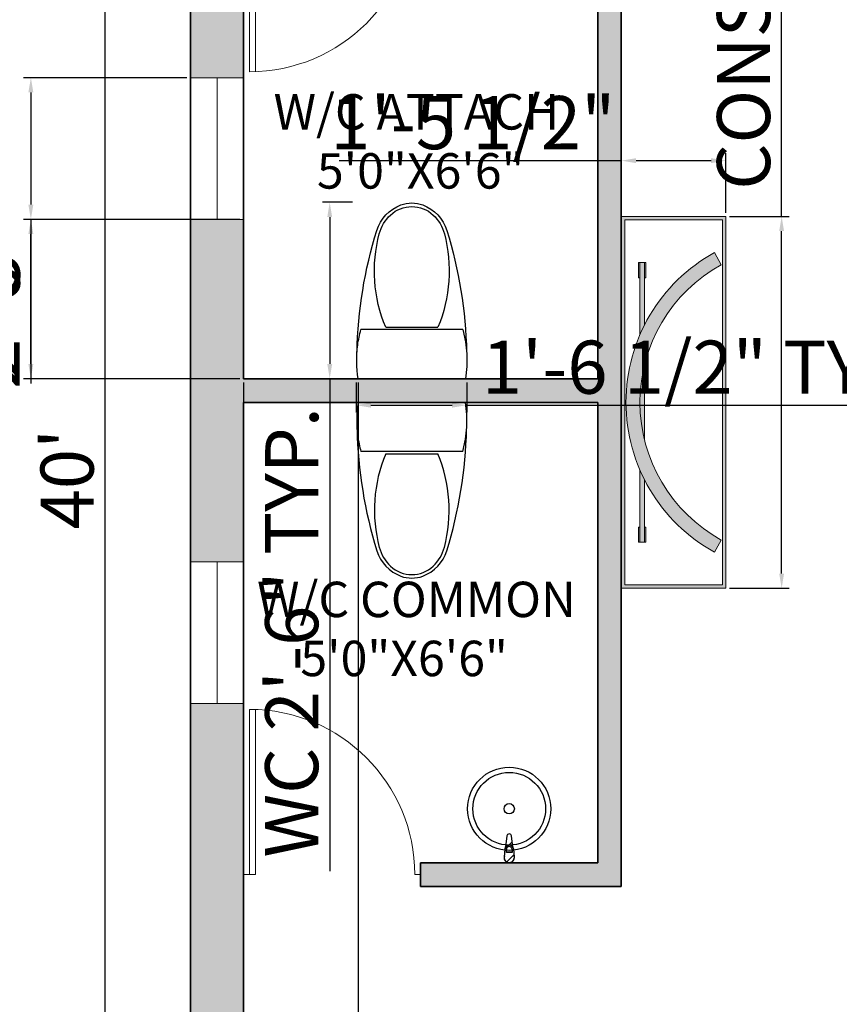
# Model space of a CAD drawing. Units: inches. Extents: x 3592 to 4861, y 1650 to 2243.
# Tile 3 of 30: x 4009 to 4148, y 1836 to 2003. Entities that reach past the tile are written whole.
import ezdxf

# ---------------------------------------------------------------- set-up
doc = ezdxf.new("R2010")
doc.units = ezdxf.units.IN
for name, color, linetype, lineweight in [('A-ANNO-DIMS', 2, 'Continuous', 13), ('A-AREA-IDEN', 7, 'Continuous', 18), ('A-DOOR', 3, 'Continuous', 20), ('A-FURN', 9, 'Continuous', 13), ('A-GLAZ', 4, 'Continuous', 18), ('A-WALL', 7, 'Continuous', 35), ('aparador', 36, 'Continuous', 9), ('moveis', 254, 'Continuous', 5), ('Сантехника', 9, 'Continuous', 18)]:
    doc.layers.add(name, color=color, linetype=linetype, lineweight=lineweight)
doc.layers.add('A-WALL-PATT', color=252, linetype='Continuous', lineweight=13, true_color=0x939598)
doc.layers.add('SANTEH', color=7, linetype='Continuous')
doc.styles.get("Standard").update_dxf_attribs({"font": 'arial.ttf'})
doc.dimstyles.new('ISO-25', dxfattribs={"dimtxt": 9, "dimasz": 2.5, "dimexe": 1.25, "dimexo": 0.625, "dimtad": 1, "dimlunit": 3, "dimtxsty": 'Standard', "dimcen": 2.5, "dimadec": 0, "dimazin": 0, "dimtfac": 1, "dimtmove": 0, "dimatfit": 3, "dimfxl": 1, "dimarcsym": 0})
pattern_1 = [(45, (-0.056, -259.036), (-35.355, 35.355), [])]

# ---------------------------------------------------------------- blocks, each defined once
blk = doc.blocks.new('2')
for p, q in [((3637.19, 1914.49), (3637.19, 1942.49)), ((3638.19, 1914.49), (3638.19, 1942.49)), ((3636.19, 1914.49), (3638.19, 1914.49)), ((3665.19, 1914.49), (3666.19, 1914.49))]:
    blk.add_line(p, q)
blk.add_arc((3637.19, 1914.49), 28, 0, 90)
blk = doc.blocks.new('*D6')
at = {"layer": 'A-ANNO-DIMS', "color": 0, "lineweight": -2, "transparency": 16777216}
for p, q in [((4037.74, 2165.22), (4022.59, 2165.22)), ((4023.84, 2162.72), (4023.84, 1687.72)), ((4037.74, 1685.22), (4022.59, 1685.22))]:
    blk.add_line(p, q, dxfattribs=at)
at = {"layer": 'A-ANNO-DIMS', "color": 0, "transparency": 16777216}
for points in [[(4023.43, 2162.72), (4024.26, 2162.72), (4023.84, 2165.22)], [(4023.43, 1687.72), (4024.26, 1687.72), (4023.84, 1685.22)]]:
    blk.add_solid(points, dxfattribs=at)
at = {"layer": 'Defpoints', "color": 0, "transparency": 16777216}
for p in [(4038.37, 2165.22), (4023.84, 1685.22), (4038.37, 1685.22)]:
    blk.add_point(p, dxfattribs=at)
at = {"layer": 'A-ANNO-DIMS', "color": 0, "transparency": 16777216, "insert": (4018.62, 1925.22), "char_height": 9, "attachment_point": 5, "rotation": 90}
blk.add_mtext("40'", dxfattribs=at)
blk = doc.blocks.new('r13')
at = {"layer": 'SANTEH', "ltscale": 5}
h = blk.add_hatch(dxfattribs=at)
h.set_pattern_fill('100__1', color=256, scale=0.5, angle=45, style=0)
h.set_pattern_definition(pattern_1)
h.paths.add_polyline_path([(-0.1, -138.2, -0.378173), (-11.2, -128.4), (-17.8, -75.5, -0.12102), (-21.1, -66), (-23.4, -32.9, -0.524536), (-0.1, 1)], flags=0)
h = blk.add_hatch(dxfattribs=at)
h.set_pattern_fill('100__1', color=256, scale=0.5, angle=45, style=0)
h.set_pattern_definition(pattern_1)
h.paths.add_polyline_path([(-0.1, -138.2, 0.378173), (11, -128.4), (17.7, -75.5, 0.12102), (20.9, -66), (23.3, -32.9, 0.524536), (-0.1, 1)], flags=0)
for p, q in [((-24, -25.7), (-23.9, -20.6)), ((-21.1, -66), (-24, -25.7)), ((20.9, -66), (23.8, -25.7)), ((23.8, -25.7), (23.8, -20.7)), ((-17.8, -75.5), (-11.2, -128.4)), ((-13.7, -48.9), (13.5, -48.9)), ((-13.7, -63.8), (-13.7, -48.9)), ((-13.7, -49.6), (13.5, -49.6)), ((11, -128.4), (17.7, -75.5)), ((13.5, -48.9), (13.5, -63.8))]:
    blk.add_line(p, q, dxfattribs=at)
for radius in [200, 175, 25]:
    blk.add_circle((-0.1, -259), radius, dxfattribs=at)
for centre, radius, start, end in [((-0.1, -24), 25, 339.2856, 200.7144), ((-0.1, -24), 24, 7.8374, 171.8967), ((-0.1, -63.4), 21.1, 185.1696, 354.8304), ((-0.1, -64.1), 21.1, 185.1696, 354.8304), ((-0.1, -63.8), 13.6, 180, 0), ((-0.1, -127), 11.2, 187.1389, 352.8611)]:
    blk.add_arc(centre, radius, start, end, dxfattribs=at)
blk = doc.blocks.new('y5')
at = {"layer": 'SANTEH', "ltscale": 5}
for p, q in [((392.5, 0), (0, 0)), ((382.5, -180), (10, -180)), ((100.6, -188.2), (291.9, -188.2))]:
    blk.add_line(p, q, dxfattribs=at)
blk.add_lwpolyline([(382.5, -180), (392.6, -134.7), (397.5, -90.9), (397.5, -44.6), (392.5, 0)], dxfattribs=at)
for centre, radius, start, end in [((406.3, -67.7), 411.9, 170.5377, 187.7399), ((1615.7, -62.7), 1620.4, 181.2224, 197.2477), ((-1223.2, -62.7), 1620.4, 342.7523, 358.7776), ((406.3, -67.7), 411.9, 187.7399, 195.822), ((594.7, -394.2), 535.3, 157.3737, 194.7786), ((-202.2, -394.2), 535.3, 345.2214, 22.6263), ((216.9, -493.8), 144.6, 194.7786, 226.8543), ((175.6, -493.8), 144.6, 313.1457, 345.2214), ((207.1, -500), 145.4, 197.2477, 249.5476), ((185.4, -500), 145.4, 290.4524, 342.7523), ((196.3, -515.9), 114.4, 226.8543, 313.1457), ((196.3, -529), 114.4, 249.5476, 290.4524)]:
    blk.add_arc(centre, radius, start, end, dxfattribs=at)
blk = doc.blocks.new('Aparador ORGANICA Formatto')
at = {"layer": 'aparador', "ltscale": 0.3}
h = blk.add_hatch(color=256, dxfattribs=at)
h.dxf.hatch_style = 1
h.set_gradient(color1=(118, 213, 123), color2=(52, 168, 57), one_color=1, tint=0.43, name='INVCURVED')
h.paths.add_polyline_path([(0.8, 0.45), (-0.8, 0.45), (-0.8, 0), (0.8, 0)])
h.paths.add_polyline_path([(0.785, 0.435), (0.785, 0.015), (-0.785, 0.015), (-0.785, 0.435)], flags=16)
h.paths.add_polyline_path([(0.2911, 0.3699), (0.5365, 0.3699), (0.5365, 0.3757), (0.6011, 0.3757), (0.6011, 0.3699), (0.6011, 0.3499), (0.6011, 0.3441), (0.5365, 0.3441), (0.5365, 0.3499), (0.3338, 0.3499, -0.150336), (0.6449, 0.0488), (0.5923, 0.0199, 0.208852), (0.1632, 0.3499), (-0.1632, 0.3499, 0.208852), (-0.5923, 0.0199), (-0.6449, 0.0488, -0.150336), (-0.3338, 0.3499), (-0.5365, 0.3499), (-0.5365, 0.3441), (-0.6011, 0.3441), (-0.6011, 0.3499), (-0.6011, 0.3699), (-0.6011, 0.3757), (-0.5365, 0.3757), (-0.5365, 0.3699), (-0.2911, 0.3699, -0.206106)], flags=0)
h = blk.add_hatch(color=256, dxfattribs=at)
h.dxf.hatch_style = 1
h.set_gradient(color1=(135, 92, 69), color2=(0, 0, 0), one_color=1, name='INVCURVED')
h.paths.add_polyline_path([(-0.6449, 0.0488), (-0.5923, 0.0199, -0.590888), (0.5923, 0.0199), (0.6449, 0.0488, 0.590888)])
h = blk.add_hatch(color=256, dxfattribs=at)
h.dxf.hatch_style = 1
h.set_gradient(color1=(178, 189, 189), one_color=1, tint=1, name='CYLINDER')
h.paths.add_polyline_path([(-0.5365, 0.3757), (-0.6011, 0.3757), (-0.6011, 0.3699), (-0.5365, 0.3699)])
h.paths.add_polyline_path([(-0.5365, 0.3499), (-0.6011, 0.3499), (-0.6011, 0.3441), (-0.5365, 0.3441)])
h = blk.add_hatch(color=256, dxfattribs=at)
h.dxf.hatch_style = 1
h.set_gradient(color1=(118, 213, 123), color2=(31, 101, 35), one_color=1, tint=0.26, name='INVCURVED')
h.paths.add_polyline_path([(-0.2911, 0.3699), (-0.6011, 0.3699), (-0.6011, 0.3499), (-0.3338, 0.3499, -0.015999)])
h = blk.add_hatch(color=256, dxfattribs=at)
h.dxf.hatch_style = 1
h.set_gradient(color1=(118, 213, 123), color2=(31, 101, 35), one_color=1, tint=0.26, name='INVCURVED')
h.paths.add_polyline_path([(-0.1632, 0.3499), (0.1632, 0.3499, 0.122516)])
h = blk.add_hatch(color=256, dxfattribs=at)
h.dxf.hatch_style = 1
h.set_gradient(color1=(118, 213, 123), color2=(31, 101, 35), one_color=1, tint=0.26, name='INVCURVED')
h.paths.add_polyline_path([(0.6011, 0.3699), (0.2911, 0.3699, -0.015999), (0.3338, 0.3499), (0.6011, 0.3499)])
h = blk.add_hatch(color=256, dxfattribs=at)
h.dxf.hatch_style = 1
h.set_gradient(color1=(178, 189, 189), one_color=1, tint=1, name='CYLINDER')
h.paths.add_polyline_path([(0.6011, 0.3757), (0.5365, 0.3757), (0.5365, 0.3699), (0.6011, 0.3699)])
h.paths.add_polyline_path([(0.6011, 0.3499), (0.5365, 0.3499), (0.5365, 0.3441), (0.6011, 0.3441)])
for p, q in [((-0.5923, 0.0199), (-0.6449, 0.0488)), ((0.5923, 0.0199), (0.6449, 0.0488))]:
    blk.add_line(p, q, dxfattribs=at)
for points in [[(-0.6011, 0.3699), (-0.6011, 0.3757), (-0.5365, 0.3757), (-0.5365, 0.3699)], [(-0.5365, 0.3499), (-0.5365, 0.3441), (-0.6011, 0.3441), (-0.6011, 0.3499)], [(0.6011, 0.3699), (0.6011, 0.3757), (0.5365, 0.3757), (0.5365, 0.3699)], [(0.5365, 0.3499), (0.5365, 0.3441), (0.6011, 0.3441), (0.6011, 0.3499)]]:
    blk.add_lwpolyline(points, dxfattribs=at)
for radius in [0.7362, 0.6762]:
    blk.add_arc((0, -0.3063), radius, 28.8434, 151.1566, dxfattribs=at)
at = {"layer": 'moveis', "ltscale": 0.3}
for p, q in [((-0.6011, 0.3699), (-0.6011, 0.3499)), ((-0.2911, 0.3699), (-0.6011, 0.3699)), ((-0.6011, 0.3499), (-0.3338, 0.3499)), ((-0.1632, 0.3499), (0.1632, 0.3499)), ((0.2911, 0.3699), (0.6011, 0.3699)), ((0.6011, 0.3499), (0.3338, 0.3499)), ((0.6011, 0.3699), (0.6011, 0.3499))]:
    blk.add_line(p, q, dxfattribs=at)
for points in [[(-0.8, 0), (0.8, 0), (0.8, 0.45), (-0.8, 0.45)], [(-0.785, 0.015), (0.785, 0.015), (0.785, 0.435), (-0.785, 0.435)]]:
    blk.add_lwpolyline(points, close=True, dxfattribs=at)
blk = doc.blocks.new('*D142')
at = {"layer": 'A-ANNO-DIMS', "color": 0, "lineweight": -2, "transparency": 16777216}
for p, q in [((3886.06, 2021.59), (3886.06, 2014.67)), ((3928.06, 2021.59), (3928.06, 2014.67)), ((3888.56, 2015.92), (3925.56, 2015.92)), ((3928.06, 2015.92), (4082.63, 2015.92))]:
    blk.add_line(p, q, dxfattribs=at)
at = {"layer": 'A-ANNO-DIMS', "color": 0, "transparency": 16777216}
for points in [[(3888.56, 2016.34), (3888.56, 2015.5), (3886.06, 2015.92)], [(3925.56, 2016.34), (3925.56, 2015.5), (3928.06, 2015.92)]]:
    blk.add_solid(points, dxfattribs=at)
at = {"layer": 'Defpoints', "color": 0, "transparency": 16777216}
for p in [(3886.06, 2022.22), (3928.06, 2022.22), (3928.06, 2015.92)]:
    blk.add_point(p, dxfattribs=at)
at = {"layer": 'A-ANNO-DIMS', "color": 0, "transparency": 16777216, "insert": (4006.6, 2021.2), "char_height": 9, "attachment_point": 5}
blk.add_mtext('DOUBLE DOOR 3\'-6" TYP.', dxfattribs=at)
blk = doc.blocks.new('*D152')
at = {"layer": 'A-ANNO-DIMS', "color": 0, "lineweight": -2, "transparency": 16777216}
for p, q in [((4065.82, 1972.11), (4060.71, 1972.11)), ((4061.96, 1969.61), (4061.96, 1944.72)), ((4065.82, 1942.22), (4060.71, 1942.22)), ((4061.96, 1942.22), (4061.96, 1858.8))]:
    blk.add_line(p, q, dxfattribs=at)
at = {"layer": 'A-ANNO-DIMS', "color": 0, "transparency": 16777216}
for points in [[(4061.55, 1969.61), (4062.38, 1969.61), (4061.96, 1972.11)], [(4061.55, 1944.72), (4062.38, 1944.72), (4061.96, 1942.22)]]:
    blk.add_solid(points, dxfattribs=at)
at = {"layer": 'Defpoints', "color": 0, "transparency": 16777216}
for p in [(4066.45, 1972.11), (4061.96, 1942.22), (4066.45, 1942.22)]:
    blk.add_point(p, dxfattribs=at)
at = {"layer": 'A-ANNO-DIMS', "color": 0, "transparency": 16777216, "insert": (4056.68, 1899.26), "char_height": 9, "attachment_point": 5, "rotation": 90}
blk.add_mtext('WC 2\'-6" TYP.', dxfattribs=at)
blk = doc.blocks.new('*D153')
at = {"layer": 'A-ANNO-DIMS', "color": 0, "lineweight": -2, "transparency": 16777216}
for p, q in [((4066.45, 1941.59), (4066.45, 1936.49)), ((4085.18, 1941.59), (4085.18, 1936.49)), ((4068.95, 1937.74), (4082.68, 1937.74)), ((4085.18, 1937.74), (4163.92, 1937.74))]:
    blk.add_line(p, q, dxfattribs=at)
at = {"layer": 'A-ANNO-DIMS', "color": 0, "transparency": 16777216}
for points in [[(4068.95, 1938.15), (4068.95, 1937.32), (4066.45, 1937.74)], [(4082.68, 1938.15), (4082.68, 1937.32), (4085.18, 1937.74)]]:
    blk.add_solid(points, dxfattribs=at)
at = {"layer": 'Defpoints', "color": 0, "transparency": 16777216}
for p in [(4066.45, 1942.22), (4085.18, 1942.22), (4085.18, 1937.74)]:
    blk.add_point(p, dxfattribs=at)
at = {"layer": 'A-ANNO-DIMS', "color": 0, "transparency": 16777216, "insert": (4125.8, 1943.01), "char_height": 9, "attachment_point": 5}
blk.add_mtext('1\'-6 1/2" TYP.', dxfattribs=at)
blk = doc.blocks.new('*D168')
at = {"layer": 'A-ANNO-DIMS', "color": 0, "lineweight": -2, "transparency": 16777216}
for p, q in [((4138.54, 1969.72), (4138.54, 2062.26)), ((4129.71, 1969.72), (4139.79, 1969.72)), ((4138.54, 1909.22), (4138.54, 1967.22)), ((4129.71, 1906.72), (4139.79, 1906.72))]:
    blk.add_line(p, q, dxfattribs=at)
at = {"layer": 'A-ANNO-DIMS', "color": 0, "transparency": 16777216}
for points in [[(4138.12, 1967.22), (4138.95, 1967.22), (4138.54, 1969.72)], [(4138.12, 1909.22), (4138.95, 1909.22), (4138.54, 1906.72)]]:
    blk.add_solid(points, dxfattribs=at)
at = {"layer": 'Defpoints', "color": 0, "transparency": 16777216}
for p in [(4129.09, 1969.72), (4138.54, 1969.72), (4129.09, 1906.72)]:
    blk.add_point(p, dxfattribs=at)
at = {"layer": 'A-ANNO-DIMS', "color": 0, "transparency": 16777216, "insert": (4133.25, 2017.24), "char_height": 9, "attachment_point": 5, "rotation": 90}
blk.add_mtext('CONSOLE 5\'-3"', dxfattribs=at)
blk = doc.blocks.new('*D169')
at = {"layer": 'A-ANNO-DIMS', "color": 0, "lineweight": -2, "transparency": 16777216}
for p, q in [((4111.37, 1970.34), (4111.37, 1980.41)), ((4129.09, 1970.34), (4129.09, 1980.41)), ((4111.37, 1979.16), (4063.57, 1979.16)), ((4126.59, 1979.16), (4113.87, 1979.16))]:
    blk.add_line(p, q, dxfattribs=at)
at = {"layer": 'A-ANNO-DIMS', "color": 0, "transparency": 16777216}
for points in [[(4113.87, 1979.58), (4113.87, 1978.75), (4111.37, 1979.16)], [(4126.59, 1979.58), (4126.59, 1978.75), (4129.09, 1979.16)]]:
    blk.add_solid(points, dxfattribs=at)
at = {"layer": 'Defpoints', "color": 0, "transparency": 16777216}
for p in [(4111.37, 1979.16), (4111.37, 1969.72), (4129.09, 1969.72)]:
    blk.add_point(p, dxfattribs=at)
at = {"layer": 'A-ANNO-DIMS', "color": 0, "transparency": 16777216, "insert": (4086.22, 1984.44), "char_height": 9, "attachment_point": 5}
blk.add_mtext('1\'-5 1/2"', dxfattribs=at)
blk = doc.blocks.new('*D174')
at = {"layer": 'A-ANNO-DIMS', "color": 0, "lineweight": -2, "transparency": 16777216}
for p, q in [((4037.74, 1993.22), (4010.07, 1993.22)), ((4011.32, 1990.72), (4011.32, 1971.72)), ((4037.74, 1969.22), (4010.07, 1969.22)), ((4011.32, 1969.22), (4011.32, 1941.39))]:
    blk.add_line(p, q, dxfattribs=at)
at = {"layer": 'A-ANNO-DIMS', "color": 0, "transparency": 16777216}
for points in [[(4010.9, 1990.72), (4011.74, 1990.72), (4011.32, 1993.22)], [(4010.9, 1971.72), (4011.74, 1971.72), (4011.32, 1969.22)]]:
    blk.add_solid(points, dxfattribs=at)
at = {"layer": 'Defpoints', "color": 0, "transparency": 16777216}
for p in [(4038.37, 1993.22), (4011.32, 1969.22), (4038.37, 1969.22)]:
    blk.add_point(p, dxfattribs=at)
at = {"layer": 'A-ANNO-DIMS', "color": 0, "transparency": 16777216, "insert": (4006.1, 1954.06), "char_height": 9, "attachment_point": 5, "rotation": 90}
blk.add_mtext('2\'-0"', dxfattribs=at)
blk = doc.blocks.new('*D175')
at = {"layer": 'A-ANNO-DIMS', "color": 0, "lineweight": -2, "transparency": 16777216}
for p, q in [((4046.74, 1969.22), (4010.07, 1969.22)), ((4011.32, 1944.72), (4011.32, 1966.72)), ((4046.74, 1942.22), (4010.07, 1942.22))]:
    blk.add_line(p, q, dxfattribs=at)
at = {"layer": 'A-ANNO-DIMS', "color": 0, "transparency": 16777216}
for points in [[(4010.9, 1966.72), (4011.74, 1966.72), (4011.32, 1969.22)], [(4010.9, 1944.72), (4011.74, 1944.72), (4011.32, 1942.22)]]:
    blk.add_solid(points, dxfattribs=at)
at = {"layer": 'Defpoints', "color": 0, "transparency": 16777216}
for p in [(4011.32, 1969.22), (4047.37, 1969.22), (4047.37, 1942.22)]:
    blk.add_point(p, dxfattribs=at)
at = {"layer": 'A-ANNO-DIMS', "color": 0, "transparency": 16777216, "insert": (4006.1, 1955.72), "char_height": 9, "attachment_point": 5, "rotation": 90}
blk.add_mtext('2\'-3"', dxfattribs=at)
blk = doc.blocks.new('*D178')
at = {"layer": 'A-ANNO-DIMS', "color": 0, "lineweight": -2, "transparency": 16777216}
for p, q in [((4047.37, 1941.59), (4047.37, 1656.92)), ((4066.79, 1941.59), (4066.79, 1656.92)), ((4049.87, 1658.17), (4064.29, 1658.17)), ((4066.79, 1658.17), (4114.59, 1658.17))]:
    blk.add_line(p, q, dxfattribs=at)
at = {"layer": 'A-ANNO-DIMS', "color": 0, "transparency": 16777216}
for points in [[(4049.87, 1658.59), (4049.87, 1657.75), (4047.37, 1658.17)], [(4064.29, 1658.59), (4064.29, 1657.75), (4066.79, 1658.17)]]:
    blk.add_solid(points, dxfattribs=at)
at = {"layer": 'Defpoints', "color": 0, "transparency": 16777216}
for p in [(4047.37, 1942.22), (4066.79, 1942.22), (4066.79, 1658.17)]:
    blk.add_point(p, dxfattribs=at)
at = {"layer": 'A-ANNO-DIMS', "color": 0, "transparency": 16777216, "insert": (4091.94, 1663.45), "char_height": 9, "attachment_point": 5}
blk.add_mtext('1\'-7 1/2"', dxfattribs=at)

msp = doc.modelspace()

# ---------------------------------------------------------------- hatches: boundary and pattern name
at = {"layer": 'A-WALL-PATT'}
h = msp.add_hatch(color=256, dxfattribs=at)
h.dxf.hatch_style = 1
h.paths.add_polyline_path([(4398.37, 2165.219), (4038.37, 2165.219), (4038.37, 1993.219), (4047.37, 1993.219), (4047.37, 2156.219), (4191.37, 2156.219), (4191.37, 2150.219), (4195.37, 2150.219), (4195.37, 2156.219), (4256.37, 2156.219), (4256.37, 2150.219), (4265.37, 2150.219), (4265.37, 2156.219), (4389.37, 2156.219), (4389.37, 2114.219), (4398.37, 2114.219)])
h.paths.add_polyline_path([(4265.37, 2102.219), (4256.37, 2102.219), (4256.37, 2096.219), (4195.37, 2096.219), (4195.37, 2102.219), (4191.37, 2102.219), (4191.37, 2020.219), (4195.37, 2020.219), (4195.37, 2087.219), (4256.37, 2087.219), (4256.37, 2020.219), (4306.37, 2020.219), (4306.37, 2024.219), (4265.37, 2024.219)], flags=17)
h.paths.add_polyline_path([(4398.37, 2066.219), (4389.37, 2066.219), (4389.37, 2024.219), (4348.37, 2024.219), (4348.37, 2020.219), (4389.37, 2020.219), (4389.37, 1989.719), (4398.37, 1989.719)])
h.paths.add_polyline_path([(4398.37, 1941.719), (4389.37, 1941.719), (4389.37, 1911.219), (4301.37, 1911.219), (4301.37, 1907.219), (4389.37, 1907.219), (4389.37, 1865.219), (4398.37, 1865.219)])
h.paths.add_polyline_path([(4398.37, 1817.219), (4389.37, 1817.219), (4389.37, 1775.219), (4265.37, 1775.219), (4265.37, 1911.219), (4256.37, 1911.219), (4256.37, 1817.219), (4220.87, 1817.219), (4220.87, 1808.219), (4256.37, 1808.219), (4256.37, 1766.219), (4389.37, 1766.219), (4389.37, 1694.219), (4256.37, 1694.219), (4256.37, 1685.219), (4398.37, 1685.219)])
h.paths.add_polyline_path([(4178.87, 1817.219), (4077.37, 1817.219), (4077.37, 1808.219), (4178.87, 1808.219)])
h.paths.add_polyline_path([(4111.37, 2020.219), (4155.37, 2020.219), (4155.37, 2024.219), (4077.37, 2024.219), (4077.37, 2020.219), (4107.37, 2020.219), (4107.37, 1942.219), (4047.37, 1942.219), (4047.37, 1969.219), (4038.37, 1969.219), (4038.37, 1911.219), (4047.37, 1911.219), (4047.37, 1938.219), (4107.37, 1938.219), (4107.37, 1860.219), (4077.37, 1860.219), (4077.37, 1856.219), (4111.37, 1856.219)])
h.paths.add_polyline_path([(4047.37, 1887.219), (4038.37, 1887.219), (4038.37, 1685.219), (4152.37, 1685.219), (4152.37, 1715.219), (4143.37, 1715.219), (4143.37, 1694.219), (4047.37, 1694.219)])
h.paths.add_polyline_path([(4152.37, 1772.219), (4143.37, 1772.219), (4143.37, 1751.219), (4152.37, 1751.219)], flags=17)

# ---------------------------------------------------------------- linework, layer by layer
at = {"layer": 'A-GLAZ'}
for p, q in [((4047.37, 1993.219), (4038.37, 1993.219)), ((4042.87, 1993.219), (4042.87, 1969.219)), ((4047.37, 1969.219), (4038.37, 1969.219)), ((4047.37, 1911.219), (4038.37, 1911.219)), ((4042.87, 1911.219), (4042.87, 1887.219)), ((4047.37, 1887.219), (4038.37, 1887.219))]:
    msp.add_line(p, q, dxfattribs=at)
at = {"layer": 'A-WALL'}
for p, q in [((4038.37, 1685.219), (4038.37, 2165.219)), ((4047.37, 1942.219), (4047.37, 2156.219)), ((4107.37, 1942.219), (4107.37, 2020.219)), ((4111.37, 1856.219), (4111.37, 2020.219)), ((4047.37, 1942.219), (4107.37, 1942.219)), ((4047.37, 1938.219), (4107.37, 1938.219)), ((4047.37, 1694.219), (4047.37, 1938.219)), ((4107.37, 1860.219), (4107.37, 1938.219)), ((4077.37, 1860.219), (4107.37, 1860.219)), ((4077.37, 1856.219), (4077.37, 1860.219)), ((4077.37, 1856.219), (4111.37, 1856.219))]:
    msp.add_line(p, q, dxfattribs=at)

# ---------------------------------------------------------------- block references
at = {"layer": 'A-DOOR', "xscale": -1, "rotation": 180}
msp.add_blockref('2', (411.181, 3936.711), dxfattribs=at)
at = {"layer": 'A-DOOR'}
msp.add_blockref('2', (411.181, -56.273), dxfattribs=at)
at = {"layer": 'A-FURN', "xscale": 39.3701, "yscale": 39.3701, "zscale": 39.3701, "rotation": 90}
msp.add_blockref('Aparador ORGANICA Formatto', (4129.086, 1938.219), dxfattribs=at)
at = {"layer": 'Сантехника', "rotation": 180}
for name, p, xscale, yscale, zscale in [('y5', (4066.788, 1942.219), -0.0462756660006946, 0.0462756660006946, 0.0462756660006946), ('r13', (4092.368, 1860.253), 0.0352097458701181, 0.0352097458701181, 0.0352097458701181)]:
    msp.add_blockref(name, p, dxfattribs=dict(at, xscale=xscale, yscale=yscale, zscale=zscale))
at = {"layer": 'Сантехника', "xscale": 0.0462756660006946, "yscale": 0.0462756660006946, "zscale": 0.0462756660006946}
msp.add_blockref('y5', (4066.788, 1938.219), dxfattribs=at)

# ---------------------------------------------------------------- texts
at = {"layer": 'A-AREA-IDEN', "char_height": 6, "attachment_point": 1}
for s, insert in [('W/C ATTACH\\P    5\'0"X6\'6"', (4052.454, 1990.429)), ('W/C COMMON\\P    5\'0"X6\'6"', (4049.648, 1907.839))]:
    msp.add_mtext_dynamic_manual_height_columns(s, width=121.44943, gutter_width=12.5, heights=[0], dxfattribs=dict(at, insert=insert))

# ---------------------------------------------------------------- dimensions: what is measured, and where the dimension line sits
at = {"layer": 'A-ANNO-DIMS'}
for base, p1, p2, angle, override, picture, middle in [((4023.842, 1685.219), (4038.37, 2165.219), (4038.37, 1685.219), 90, {"dimclrd": 0, "dimclre": 0, "dimclrt": 0}, '*D6', (4018.622, 1925.219)), ((4111.37, 1979.164), (4129.086, 1969.715), (4111.37, 1969.715), 180, {"dimdec": 1, "dimlfac": 1, "dimrnd": 0, "dimzin": 1, "dimdsep": 46, "dimlunit": 4, "dimfrac": 2}, '*D169', (4086.221, 1984.442)), ((4011.32, 1969.219), (4038.37, 1993.219), (4038.37, 1969.219), 90, {"dimdec": 1, "dimlfac": 1, "dimrnd": 0, "dimzin": 1, "dimdsep": 46, "dimlunit": 4, "dimfrac": 2}, '*D174', (4006.1, 1954.055)), ((4011.32, 1969.219), (4047.37, 1942.219), (4047.37, 1969.219), 90, {"dimdec": 1, "dimlfac": 1, "dimrnd": 0, "dimzin": 1, "dimdsep": 46, "dimlunit": 4, "dimfrac": 2}, '*D175', (4006.096, 1955.719))]:
    dim = msp.add_linear_dim(base=base, p1=p1, p2=p2, angle=angle, dimstyle='ISO-25', override=override, dxfattribs=at)
    dim.commit()
    dim.dimension.update_dxf_attribs({"geometry": picture, "text_midpoint": middle})
for base, p1, p2, angle, text, picture, middle in [((4138.535, 1969.715), (4129.086, 1906.723), (4129.086, 1969.715), 90, 'CONSOLE <>', '*D168', (4133.25, 2017.238)), ((4061.962, 1942.219), (4066.445, 1972.106), (4066.445, 1942.219), 270, 'WC <> TYP.', '*D152', (4056.684, 1899.26))]:
    dim = msp.add_linear_dim(base=base, p1=p1, p2=p2, angle=angle, text=text, dimstyle='ISO-25', override={"dimdec": 1, "dimlfac": 1, "dimrnd": 0, "dimzin": 1, "dimdsep": 46, "dimlunit": 4, "dimfrac": 2}, dxfattribs=at)
    dim.commit()
    dim.dimension.update_dxf_attribs({"geometry": picture, "text_midpoint": middle})
for base, p1, p2, text, picture, middle in [((3928.061, 2015.919), (3886.061, 2022.219), (3928.061, 2022.219), 'DOUBLE DOOR <> TYP.', '*D142', (4006.597, 2021.204)), ((4085.182, 1937.736), (4066.445, 1942.219), (4085.182, 1942.219), '<> TYP.', '*D153', (4125.799, 1943.014))]:
    dim = msp.add_linear_dim(base=base, p1=p1, p2=p2, text=text, dimstyle='ISO-25', override={"dimdec": 1, "dimlfac": 1, "dimrnd": 0, "dimzin": 1, "dimdsep": 46, "dimlunit": 4, "dimfrac": 2}, dxfattribs=at)
    dim.commit()
    dim.dimension.update_dxf_attribs({"geometry": picture, "text_midpoint": middle})
dim = msp.add_linear_dim(base=(4066.788, 1658.169), p1=(4047.37, 1942.219), p2=(4066.788, 1942.219), dimstyle='ISO-25', override={"dimdec": 1, "dimlfac": 1, "dimrnd": 0, "dimzin": 1, "dimdsep": 46, "dimlunit": 4, "dimfrac": 2}, dxfattribs=at)
dim.commit()
dim.dimension.update_dxf_attribs({"geometry": '*D178', "text_midpoint": (4091.938, 1663.447)})

doc.saveas('drawing.dxf')
